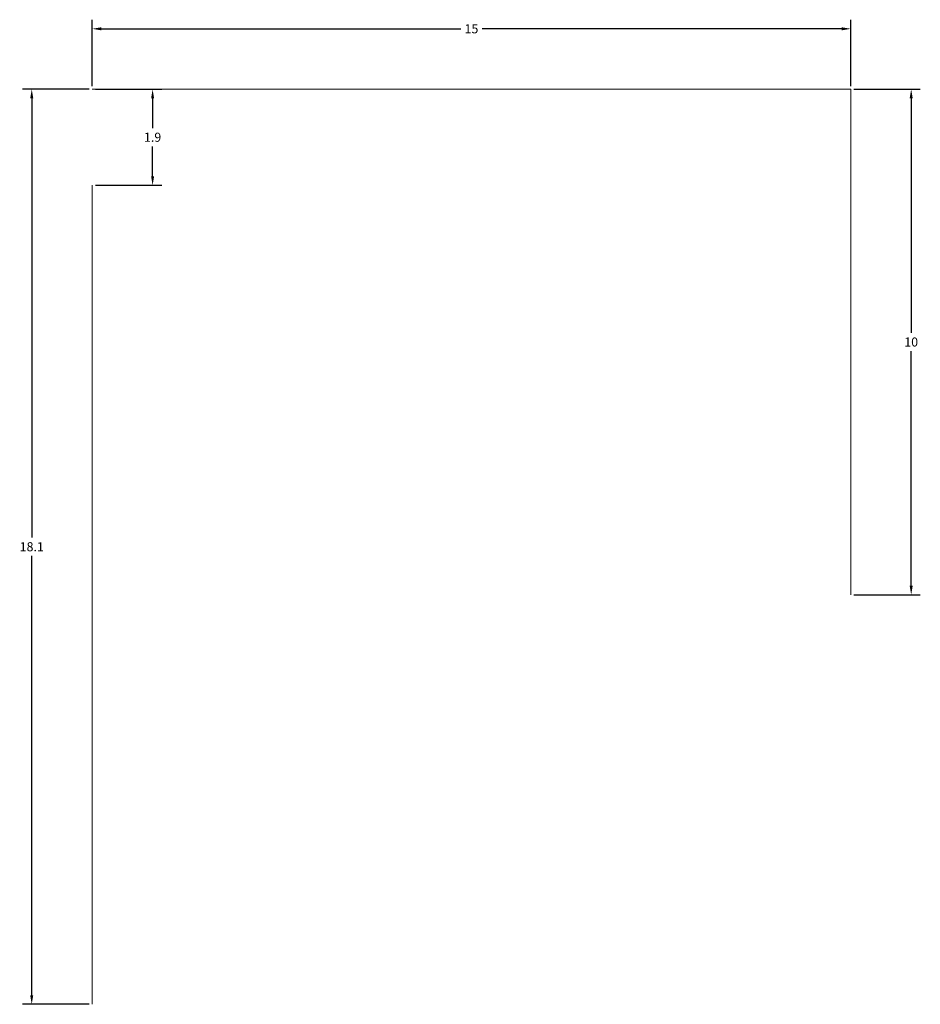
# Model space of a CAD drawing. Units: inches. Extents: x 944.1 to 961.9, y -18.1 to 1.4.
import ezdxf

# ---------------------------------------------------------------- set-up
doc = ezdxf.new("R2010")
doc.units = ezdxf.units.IN
doc.header["$MEASUREMENT"] = 0
doc.layers.add('M-CONS', color=8, linetype='Continuous', lineweight=18)
doc.layers.add('M-DIMS', color=2, linetype='Continuous', lineweight=18)
doc.styles.get("Standard").update_dxf_attribs({"font": 'arial.ttf'})
doc.dimstyles.get("Standard").update_dxf_attribs({"dimtxt": 0.18, "dimasz": 0.18, "dimexe": 0.18, "dimexo": 0.0625, "dimgap": 0.09, "dimtad": 0, "dimtih": 1, "dimtoh": 1, "dimdec": 4, "dimzin": 0, "dimdsep": 46, "dimtxsty": 'Standard', "dimcen": 0.09, "dimadec": 0, "dimazin": 0, "dimtfac": 1, "dimtdec": 4, "dimtofl": 0, "dimtmove": 0, "dimatfit": 3, "dimfxl": 1, "dimtolj": 1, "dimtzin": 0, "dimarcsym": 0})

# ---------------------------------------------------------------- blocks, each defined once
blk = doc.blocks.new('*D1')
at = {"layer": 'Defpoints', "color": 0, "transparency": 16777216}
for p in [(960.524, 1.195), (945.524, 0), (960.524, 0)]:
    blk.add_point(p, dxfattribs=at)
at = {"layer": 'M-DIMS', "color": 0, "lineweight": -2, "transparency": 16777216}
for p, q in [((945.524, 0.062), (945.524, 1.375)), ((960.524, 0.062), (960.524, 1.375)), ((945.704, 1.195), (952.813, 1.195)), ((960.344, 1.195), (953.235, 1.195))]:
    blk.add_line(p, q, dxfattribs=at)
at = {"layer": 'M-DIMS', "color": 0, "transparency": 16777216}
for points in [[(945.704, 1.225), (945.704, 1.165), (945.524, 1.195)], [(960.344, 1.225), (960.344, 1.165), (960.524, 1.195)]]:
    blk.add_solid(points, dxfattribs=at)
at = {"layer": 'M-DIMS', "color": 0, "transparency": 16777216, "insert": (953.024, 1.195), "char_height": 0.18, "attachment_point": 5}
blk.add_mtext('\\A1;15', dxfattribs=at)
blk = doc.blocks.new('*D2')
at = {"layer": 'Defpoints', "color": 0, "transparency": 16777216}
for p in [(945.524, 0), (945.524, -1.9), (946.719, -1.9)]:
    blk.add_point(p, dxfattribs=at)
at = {"layer": 'M-DIMS', "color": 0, "lineweight": -2, "transparency": 16777216}
for p, q in [((945.587, 0), (946.899, 0)), ((946.719, -0.18), (946.719, -0.768)), ((946.719, -1.72), (946.719, -1.132)), ((945.587, -1.9), (946.899, -1.9))]:
    blk.add_line(p, q, dxfattribs=at)
at = {"layer": 'M-DIMS', "color": 0, "transparency": 16777216}
for points in [[(946.689, -0.18), (946.749, -0.18), (946.719, 0)], [(946.689, -1.72), (946.749, -1.72), (946.719, -1.9)]]:
    blk.add_solid(points, dxfattribs=at)
at = {"layer": 'M-DIMS', "color": 0, "transparency": 16777216, "insert": (946.719, -0.95), "char_height": 0.18, "attachment_point": 5}
blk.add_mtext('\\A1;1.9', dxfattribs=at)
blk = doc.blocks.new('*D3')
at = {"layer": 'Defpoints', "color": 0, "transparency": 16777216}
for p in [(945.524, 0), (944.329, 0), (945.524, -18.1)]:
    blk.add_point(p, dxfattribs=at)
at = {"layer": 'M-DIMS', "color": 0, "lineweight": -2, "transparency": 16777216}
for p, q in [((945.462, 0), (944.149, 0)), ((944.329, -0.18), (944.329, -8.868)), ((944.329, -17.92), (944.329, -9.232)), ((945.462, -18.1), (944.149, -18.1))]:
    blk.add_line(p, q, dxfattribs=at)
at = {"layer": 'M-DIMS', "color": 0, "transparency": 16777216}
for points in [[(944.299, -0.18), (944.359, -0.18), (944.329, 0)], [(944.299, -17.92), (944.359, -17.92), (944.329, -18.1)]]:
    blk.add_solid(points, dxfattribs=at)
at = {"layer": 'M-DIMS', "color": 0, "transparency": 16777216, "insert": (944.329, -9.05), "char_height": 0.18, "attachment_point": 5}
blk.add_mtext('\\A1;18.1', dxfattribs=at)
blk = doc.blocks.new('*D4')
at = {"layer": 'Defpoints', "color": 0, "transparency": 16777216}
for p in [(960.524, 0), (961.719, 0), (960.524, -10)]:
    blk.add_point(p, dxfattribs=at)
at = {"layer": 'M-DIMS', "color": 0, "lineweight": -2, "transparency": 16777216}
for p, q in [((960.587, 0), (961.899, 0)), ((961.719, -0.18), (961.719, -4.818)), ((961.719, -9.82), (961.719, -5.182)), ((960.587, -10), (961.899, -10))]:
    blk.add_line(p, q, dxfattribs=at)
at = {"layer": 'M-DIMS', "color": 0, "transparency": 16777216}
for points in [[(961.689, -0.18), (961.749, -0.18), (961.719, 0)], [(961.689, -9.82), (961.749, -9.82), (961.719, -10)]]:
    blk.add_solid(points, dxfattribs=at)
at = {"layer": 'M-DIMS', "color": 0, "transparency": 16777216, "insert": (961.719, -5), "char_height": 0.18, "attachment_point": 5}
blk.add_mtext('\\A1;10', dxfattribs=at)

msp = doc.modelspace()

# ---------------------------------------------------------------- linework, layer by layer
at = {"layer": 'M-CONS', "extrusion": (0, -1, 0)}
for p, q in [((945.524, 0, 126.945), (945.524, 0, 173.745)), ((945.524, 0, 173.745), (960.524, 0, 173.745)), ((960.524, 0, 126.945), (945.524, 0, 126.945)), ((960.524, 0, 173.745), (960.524, 0, 126.945)), ((960.524, 0, 173.745), (960.524, -10, 173.745)), ((960.524, -10, 164.549), (960.524, -10, 134.549))]:
    msp.add_line(p, q, dxfattribs=at)
at = {"layer": 'M-CONS', "extrusion": (-1, 0, 0)}
msp.add_circle((10, 150.345, -945.524), 8.1, dxfattribs=at)

# ---------------------------------------------------------------- dimensions: what is measured, and where the dimension line sits
at = {"layer": 'M-DIMS'}
dim = msp.add_linear_dim(base=(960.524, 1.195), p1=(945.524, 0), p2=(960.524, 0), dimstyle='Standard', override={"dimdec": 0, "dimlfac": 1, "dimrnd": 0, "dimzin": 0, "dimdsep": 46, "dimlunit": 2}, dxfattribs=at)
dim.commit()
dim.dimension.update_dxf_attribs({"geometry": '*D1', "text_midpoint": (953.024, 1.195)})
for base, p1, p2, angle, override, picture, middle in [((944.329, 0), (945.524, -18.1), (945.524, 0), 90, {"dimdec": 1, "dimlfac": 1, "dimrnd": 0, "dimzin": 0, "dimdsep": 46, "dimlunit": 2}, '*D3', (944.329, -9.05)), ((946.719, -1.9), (945.524, 0), (945.524, -1.9), 270, {"dimdec": 1, "dimlfac": 1, "dimrnd": 0, "dimzin": 0, "dimdsep": 46, "dimlunit": 2}, '*D2', (946.719, -0.95)), ((961.719, 0), (960.524, -10), (960.524, 0), 90, {"dimdec": 0, "dimlfac": 1, "dimrnd": 0, "dimzin": 0, "dimdsep": 46, "dimlunit": 2}, '*D4', (961.719, -5))]:
    dim = msp.add_linear_dim(base=base, p1=p1, p2=p2, angle=angle, dimstyle='Standard', override=override, dxfattribs=at)
    dim.commit()
    dim.dimension.update_dxf_attribs({"geometry": picture, "text_midpoint": middle})

doc.saveas('drawing.dxf')
